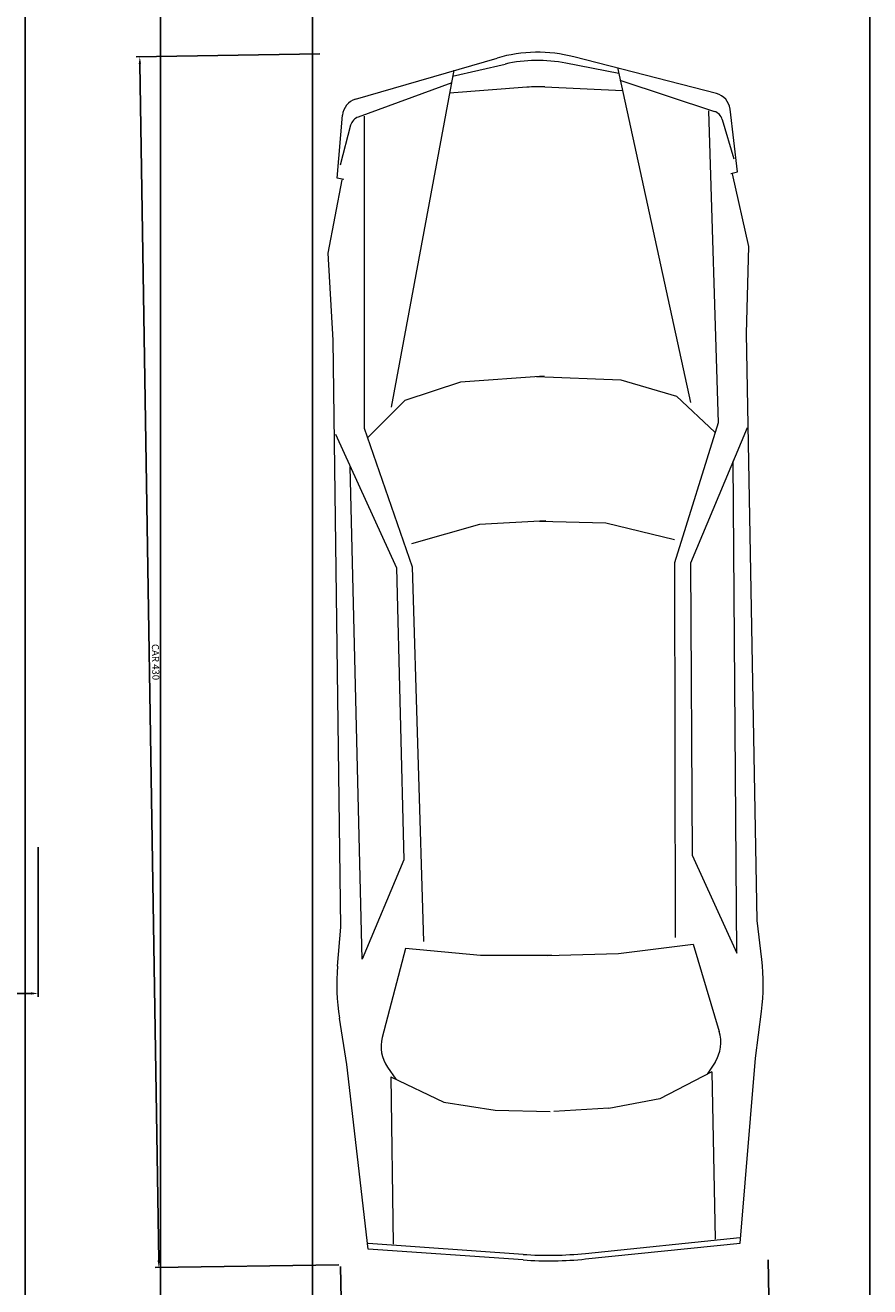
# Model space of a CAD drawing. Units: inches. Extents: x 604 to 3492, y -123 to 1737.
# Tile 4 of 20: x 1038 to 1338, y 131 to 579. Entities that reach past the tile are written whole.
import ezdxf

# ---------------------------------------------------------------- set-up
doc = ezdxf.new("R2010")
doc.units = ezdxf.units.IN
doc.layers.add('A-ANNO-DIMS', color=2, linetype='Continuous', lineweight=18)
doc.layers.add('A-SITE-VEHC', color=8, linetype='Continuous', lineweight=13)
doc.styles.get("Standard").update_dxf_attribs({"font": 'arial.ttf'})
doc.dimstyles.new('ISO-25', dxfattribs={"dimtxt": 2.5, "dimasz": 2.5, "dimexe": 1.25, "dimexo": 0.625, "dimtad": 1, "dimtxsty": 'Standard', "dimcen": 2.5, "dimadec": 0, "dimazin": 0, "dimtfac": 1, "dimtmove": 0, "dimatfit": 3, "dimfxl": 1, "dimarcsym": 0})

# ---------------------------------------------------------------- blocks, each defined once
blk = doc.blocks.new('A$C35F8349B')
for p, q in [((1.8577, 0.9043), (1.6935, 0.8881)), ((-1.4554, 0.8542), (-1.7194, 0.8273)), ((-1.4485, 0.826), (-1.4554, 0.8542)), ((-1.1403, 0.8967), (-1.4472, 0.8328)), ((-0.7743, 0.8812), (-1.1403, 0.8967)), ((1.6935, 0.8881), (-0.7742, 0.8812)), ((-0.3782, 0.8777), (0.1874, 0.6311)), ((2.2715, 0.8719), (2.0757, 0.8997)), ((3.0487, 0.7948), (2.2715, 0.8719)), ((-1.6761, 0.7938), (-1.5095, 0.84)), ((1.8294, 0.7999), (-0.2407, 0.8177)), ((1.4145, 0.6193), (1.8294, 0.7999)), ((-1.7852, 0.7717), (-1.9491, 0.1743)), ((-1.8485, 0.3655), (-1.7105, 0.7616)), ((-1.713, 0.7364), (-0.4016, 0.757)), ((-0.4016, 0.757), (0.1843, 0.5643)), ((3.0814, 0.1444), (3.0253, 0.7936)), ((3.1049, 0.1444), (3.0487, 0.7948)), ((-0.5155, 0.5838), (-0.3621, 0.7425)), ((1.7881, 0.6178), (2.1569, 0.7203)), ((2.1598, 0.7211), (2.1602, 0.7212)), ((2.2857, 0.7011), (2.3365, 0.6672)), ((2.3265, 0.6873), (3.0302, 0.6898)), ((-1.9018, 0.3573), (-0.489, 0.6422)), ((2.3265, 0.6873), (2.4359, 0.4672)), ((-0.5887, 0.3499), (-0.5155, 0.5837)), ((0.1874, 0.6311), (1.4145, 0.6193)), ((1.8224, 0.3026), (1.7881, 0.6178)), ((0.0111, 0.2787), (0.0867, 0.5657)), ((0.1843, 0.5643), (1.7599, 0.5419)), ((2.4359, 0.4672), (2.4732, 0.2515)), ((-1.8246, 0.0506), (-1.8046, 0.3763)), ((-1.8757, 0.3621), (-1.9231, 0.1408)), ((-0.6083, -0.0032), (-0.5887, 0.3499)), ((0, 0), (0.0111, 0.2787)), ((1.8263, 0.0034), (1.8224, 0.3026)), ((2.4725, 0.2515), (2.4824, 0.0204)), ((-0.6083, 0.0294), (-0.5887, -0.3237)), ((0, 0.0262), (0.0111, -0.2525)), ((1.8263, 0.0228), (1.8224, -0.2765)), ((2.4732, -0.2253), (2.4824, 0.0058)), ((-1.8246, -0.0244), (-1.8046, -0.3501)), ((-1.7852, -0.7455), (-1.9491, -0.1482)), ((-1.8757, -0.3359), (-1.9231, -0.1146)), ((3.0814, -0.1182), (3.0253, -0.7674)), ((3.1049, -0.1182), (3.0487, -0.7686)), ((0.0111, -0.2525), (0.0867, -0.5395)), ((2.4359, -0.441), (2.4732, -0.2253)), ((1.8224, -0.2765), (1.7881, -0.5916)), ((-1.9018, -0.3311), (-0.489, -0.616)), ((-1.8485, -0.3393), (-1.7105, -0.7354)), ((-0.5887, -0.3237), (-0.5155, -0.5576)), ((2.3265, -0.6611), (2.4359, -0.441)), ((0.1843, -0.5381), (1.7599, -0.5157)), ((-0.5155, -0.5576), (-0.3621, -0.7163)), ((-0.4016, -0.7308), (0.1843, -0.5381)), ((-0.3782, -0.8515), (0.1874, -0.6049)), ((0.1874, -0.6049), (1.4145, -0.5931)), ((1.4145, -0.5931), (1.8294, -0.7737)), ((1.7881, -0.5916), (2.1602, -0.695)), ((2.2857, -0.6749), (2.3365, -0.641)), ((2.3265, -0.6611), (3.0302, -0.6636)), ((-1.713, -0.7103), (-0.4016, -0.7308)), ((-1.6761, -0.7676), (-1.5095, -0.8138)), ((1.8294, -0.7737), (-0.2407, -0.7915)), ((3.0487, -0.7686), (2.2715, -0.8457)), ((-1.4554, -0.828), (-1.7194, -0.8011)), ((-1.4485, -0.7998), (-1.4554, -0.828)), ((-1.1403, -0.8705), (-1.4472, -0.8066)), ((2.2715, -0.8457), (2.0757, -0.8735)), ((-0.7742, -0.855), (-1.1403, -0.8705)), ((1.6935, -0.8619), (-0.7742, -0.855)), ((1.8577, -0.8781), (1.6935, -0.8619))]:
    blk.add_line(p, q)
for centre, radius, start, end in [((1.9473, -0.0057), 0.9144, 81.9284, 95.6257), ((-1.7117, 0.7515), 0.0762, 95.8102, 164.6615), ((-1.6625, 0.7448), 0.0508, 105.4862, 160.7894), ((2.201, 0.5744), 0.1524, 56.264, 106.8198), ((-1.3612, 0.0131), 0.6096, 164.6615, 195.3385), ((-1.327, 0.0131), 0.6096, 167.9052, 192.0948), ((1.563, 0.0131), 1.524, 355.0592, 4.9408), ((1.5866, 0.0131), 1.524, 355.0592, 4.9408), ((-1.2162, 0.0131), 0.6096, 176.4735, 183.5265), ((2.201, -0.5482), 0.1524, 254.4694, 303.7359), ((-1.6625, -0.7187), 0.0508, 199.2106, 254.5138), ((-1.7117, -0.7253), 0.0762, 195.3385, 264.1898), ((1.9473, 0.0319), 0.9144, 264.3743, 278.0716)]:
    blk.add_arc(centre, radius, start, end)
blk = doc.blocks.new('*D59')
at = {"layer": 'A-ANNO-DIMS', "color": 0, "lineweight": -2, "transparency": 16777216}
for p, q in [((678.01, 287.08), (678.01, 233.77)), ((1042.59, 287.08), (1042.59, 233.77)), ((680.51, 235.02), (1040.09, 235.02))]:
    blk.add_line(p, q, dxfattribs=at)
at = {"layer": 'A-ANNO-DIMS', "color": 0, "transparency": 16777216}
for points in [[(680.51, 235.44), (680.51, 234.61), (678.01, 235.02)], [(1040.09, 235.44), (1040.09, 234.61), (1042.59, 235.02)]]:
    blk.add_solid(points, dxfattribs=at)
at = {"layer": 'Defpoints', "color": 0, "transparency": 16777216}
for p in [(678.01, 287.7), (1042.59, 287.7), (1042.59, 235.02)]:
    blk.add_point(p, dxfattribs=at)
at = {"layer": 'A-ANNO-DIMS', "color": 0, "transparency": 16777216, "insert": (860.3, 237.15), "char_height": 2.5, "attachment_point": 5}
blk.add_mtext('364,58', dxfattribs=at)
blk = doc.blocks.new('*D81')
at = {"layer": 'A-ANNO-DIMS', "color": 0, "lineweight": -2, "transparency": 16777216}
for p, q in [((1142.63, 568.99), (1077.45, 567.97)), ((1078.74, 565.49), (1085.43, 140.11)), ((1149.4, 138.61), (1084.22, 137.59))]:
    blk.add_line(p, q, dxfattribs=at)
at = {"layer": 'A-ANNO-DIMS', "color": 0, "transparency": 16777216}
for points in [[(1079.15, 565.49), (1078.32, 565.48), (1078.7, 567.98)], [(1085.84, 140.11), (1085.01, 140.1), (1085.47, 137.61)]]:
    blk.add_solid(points, dxfattribs=at)
at = {"layer": 'Defpoints', "color": 0, "transparency": 16777216}
for p in [(1143.26, 569), (1085.47, 137.61), (1150.02, 138.62)]:
    blk.add_point(p, dxfattribs=at)
at = {"layer": 'A-ANNO-DIMS', "color": 0, "transparency": 16777216, "insert": (1084, 352.83), "char_height": 2.5, "attachment_point": 5, "rotation": 270.9007}
blk.add_mtext('CAR 430', dxfattribs=at)
blk = doc.blocks.new('*D82')
at = {"layer": 'A-ANNO-DIMS', "color": 0, "lineweight": -2, "transparency": 16777216}
for p, q in [((1301.94, 140.38), (1302.96, 75.2)), ((1150.03, 138), (1151.06, 72.81)), ((1153.54, 74.1), (1300.44, 76.41))]:
    blk.add_line(p, q, dxfattribs=at)
at = {"layer": 'A-ANNO-DIMS', "color": 0, "transparency": 16777216}
for points in [[(1300.44, 76.83), (1300.45, 76), (1302.94, 76.45)], [(1153.53, 74.52), (1153.54, 73.69), (1151.04, 74.06)]]:
    blk.add_solid(points, dxfattribs=at)
at = {"layer": 'Defpoints', "color": 0, "transparency": 16777216}
for p in [(1301.93, 141.01), (1150.02, 138.62), (1302.94, 76.45)]:
    blk.add_point(p, dxfattribs=at)
at = {"layer": 'A-ANNO-DIMS', "color": 0, "transparency": 16777216, "insert": (1226.96, 77.16), "char_height": 2.5, "attachment_point": 5, "rotation": 0.9007}
blk.add_mtext('152', dxfattribs=at)
blk = doc.blocks.new('*D86')
at = {"layer": 'A-ANNO-DIMS', "color": 0, "lineweight": -2, "transparency": 16777216}
for p, q in [((1038.01, 1272.08), (1038.01, 67.77)), ((1140.01, 1272.08), (1140.01, 67.77)), ((1040.51, 69.02), (1137.51, 69.02))]:
    blk.add_line(p, q, dxfattribs=at)
at = {"layer": 'A-ANNO-DIMS', "color": 0, "transparency": 16777216}
for points in [[(1040.51, 69.44), (1040.51, 68.61), (1038.01, 69.02)], [(1137.51, 69.44), (1137.51, 68.61), (1140.01, 69.02)]]:
    blk.add_solid(points, dxfattribs=at)
at = {"layer": 'Defpoints', "color": 0, "transparency": 16777216}
for p in [(1038.01, 1272.7), (1140.01, 1272.7), (1140.01, 69.02)]:
    blk.add_point(p, dxfattribs=at)
at = {"layer": 'A-ANNO-DIMS', "color": 0, "transparency": 16777216, "insert": (1089.01, 70.93), "char_height": 2.5, "attachment_point": 5}
blk.add_mtext('102', dxfattribs=at)
blk = doc.blocks.new('*D94')
at = {"layer": 'A-ANNO-DIMS', "color": 0, "lineweight": -2, "transparency": 16777216}
for p, q in [((1086.01, 602.08), (1086.01, 67.77)), ((1338.01, 602.08), (1338.01, 67.77)), ((1088.51, 69.02), (1335.51, 69.02))]:
    blk.add_line(p, q, dxfattribs=at)
at = {"layer": 'A-ANNO-DIMS', "color": 0, "transparency": 16777216}
for points in [[(1088.51, 69.44), (1088.51, 68.61), (1086.01, 69.02)], [(1335.51, 69.44), (1335.51, 68.61), (1338.01, 69.02)]]:
    blk.add_solid(points, dxfattribs=at)
at = {"layer": 'Defpoints', "color": 0, "transparency": 16777216}
for p in [(1086.01, 602.7), (1338.01, 602.7), (1338.01, 69.02)]:
    blk.add_point(p, dxfattribs=at)
at = {"layer": 'A-ANNO-DIMS', "color": 0, "transparency": 16777216, "insert": (1212.01, 70.93), "char_height": 2.5, "attachment_point": 5}
blk.add_mtext('252', dxfattribs=at)

msp = doc.modelspace()

# ---------------------------------------------------------------- block references
at = {"layer": 'A-SITE-VEHC', "xscale": 84.55594067420529, "yscale": 84.55594067420529, "zscale": 84.55594067420529, "rotation": 270.900724565099}
msp.add_blockref('A$C35F8349B', (1220.7307, 402.9448), dxfattribs=at)

# ---------------------------------------------------------------- dimensions: what is measured, and where the dimension line sits
at = {"layer": 'A-ANNO-DIMS'}
for base, p1, p2, override, picture, middle in [((1140.0111, 69.0242), (1038.0111, 1272.7004), (1140.0111, 1272.7004), {"dimdec": 0, "dimlfac": 1, "dimrnd": 0, "dimzin": 0, "dimdsep": 46, "dimlunit": 2}, '*D86', (1089.0111, 70.9256)), ((1338.0111, 69.0242), (1086.0111, 602.7004), (1338.0111, 602.7004), {"dimdec": 0, "dimlfac": 1, "dimrnd": 0, "dimzin": 0, "dimdsep": 46, "dimlunit": 2}, '*D94', (1212.0111, 70.9256)), ((1042.5874, 235.0232), (678.0111, 287.7004), (1042.5874, 287.7004), {"dimclrd": 0, "dimclre": 0, "dimclrt": 0}, '*D59', (860.2993, 237.1506))]:
    dim = msp.add_linear_dim(base=base, p1=p1, p2=p2, dimstyle='ISO-25', override=override, dxfattribs=at)
    dim.commit()
    dim.dimension.update_dxf_attribs({"geometry": picture, "text_midpoint": middle})
dim = msp.add_linear_dim(base=(1085.4652, 137.6055), p1=(1143.2557, 568.9999), p2=(1150.0221, 138.6204), angle=270.900725, text='CAR <>', dimstyle='ISO-25', override={"dimdec": 0, "dimlfac": 1, "dimrnd": 0, "dimzin": 0, "dimdsep": 46, "dimlunit": 2}, dxfattribs=at)
dim.commit()
dim.dimension.update_dxf_attribs({"geometry": '*D81', "text_midpoint": (1084.0003, 352.8254)})
dim = msp.add_linear_dim(base=(1302.9429, 76.4518), p1=(1150.0221, 138.6204), p2=(1301.9279, 141.0087), angle=0.900725, dimstyle='ISO-25', override={"dimdec": 0, "dimlfac": 1, "dimrnd": 0, "dimzin": 0, "dimdsep": 46, "dimlunit": 2}, dxfattribs=at)
dim.commit()
dim.dimension.update_dxf_attribs({"geometry": '*D82', "text_midpoint": (1226.9601, 77.1589)})

doc.saveas('drawing.dxf')
